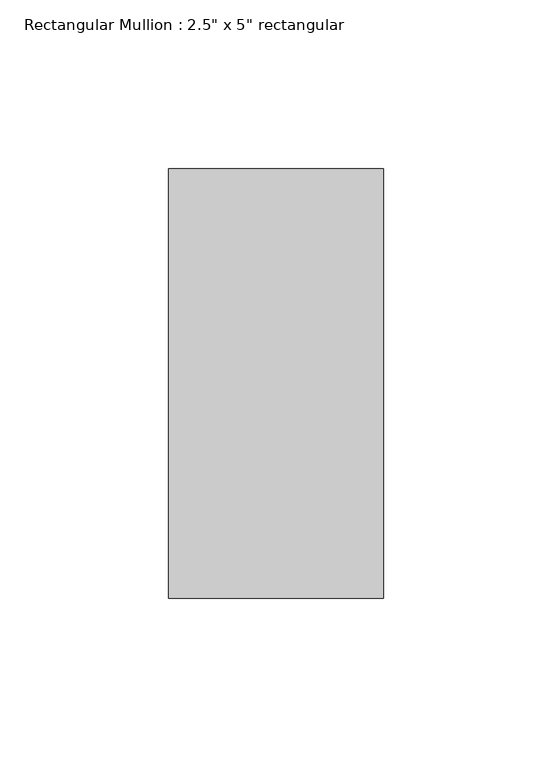
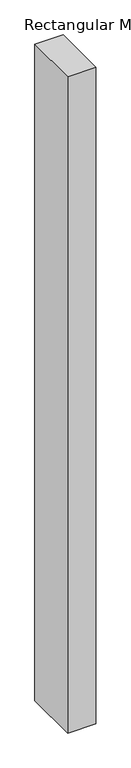
"""IFC4 building model written with IfcOpenShell, lengths in millimetres: member geometry."""

from ifc_helpers import new_model, si_unit, frame, origin, place, context, project, spatial, polyline, outline, extrude, source, transform, mapped, element, save


def member_0ab19f0c(model_context):
    return source(origin(), model_context, "Body", "SweptSolid", [
        extrude(outline(polyline([(31.75, 63.5), (31.75, -63.5), (-31.75, -63.5), (-31.75, 63.5), (31.75, 63.5)])), frame((0.0, 0.0, -1560.9513331), z_axis=(0.0, 0.0, 1.0), x_axis=(1.0, 0.0, 0.0)), (0.0, 0.0, 1.0), 1560.9513331),
    ])


if __name__ == "__main__":
    model = new_model("IFC4")
    model_context = context("Model", 3, world=origin())
    ifc_project = project(units=[si_unit("LENGTHUNIT", "METRE", prefix="MILLI")], contexts=[model_context])
    site = spatial("IfcSite", under=ifc_project)
    building = spatial("IfcBuilding", under=site)
    placement = place(None, origin())
    member_shape = member_0ab19f0c(model_context)
    element("IfcMember", 1, ObjectType="Rectangular Mullion : 2.5\" x 5\" rectangular", at=placement, inside=building, context=model_context, shape_type="MappedRepresentation", body=[
        mapped(member_shape, transform((0.0, 0.0, 0.0), x_axis=(1.0, 0.0, 0.0), y_axis=(0.0, 1.0, 0.0), z_axis=(0.0, 0.0, 1.0))),
    ])
    save(model, "model.ifc")

# Revit data of these elements
# Type "Rectangular Mullion : 2.5\" x 5\" rectangular"
#   built-in parameter 1007304 = 0.416667 (stored number, unit not read)
#   built-in parameter 1007301 = 0.104167 (stored number, unit not read)
#   built-in parameter 1007300 = 0.104167 (stored number, unit not read)
# Element 1 (IfcMember, "Rectangular Mullion : 2.5\" x 5\" rectangular")
#   Materials on its faces: "Aluminum"
# Materials
#   "Aluminum": class "Metal", colour RGB 247 247 247, transparency 0, Description = "Aluminum 6061", Cost = 0
